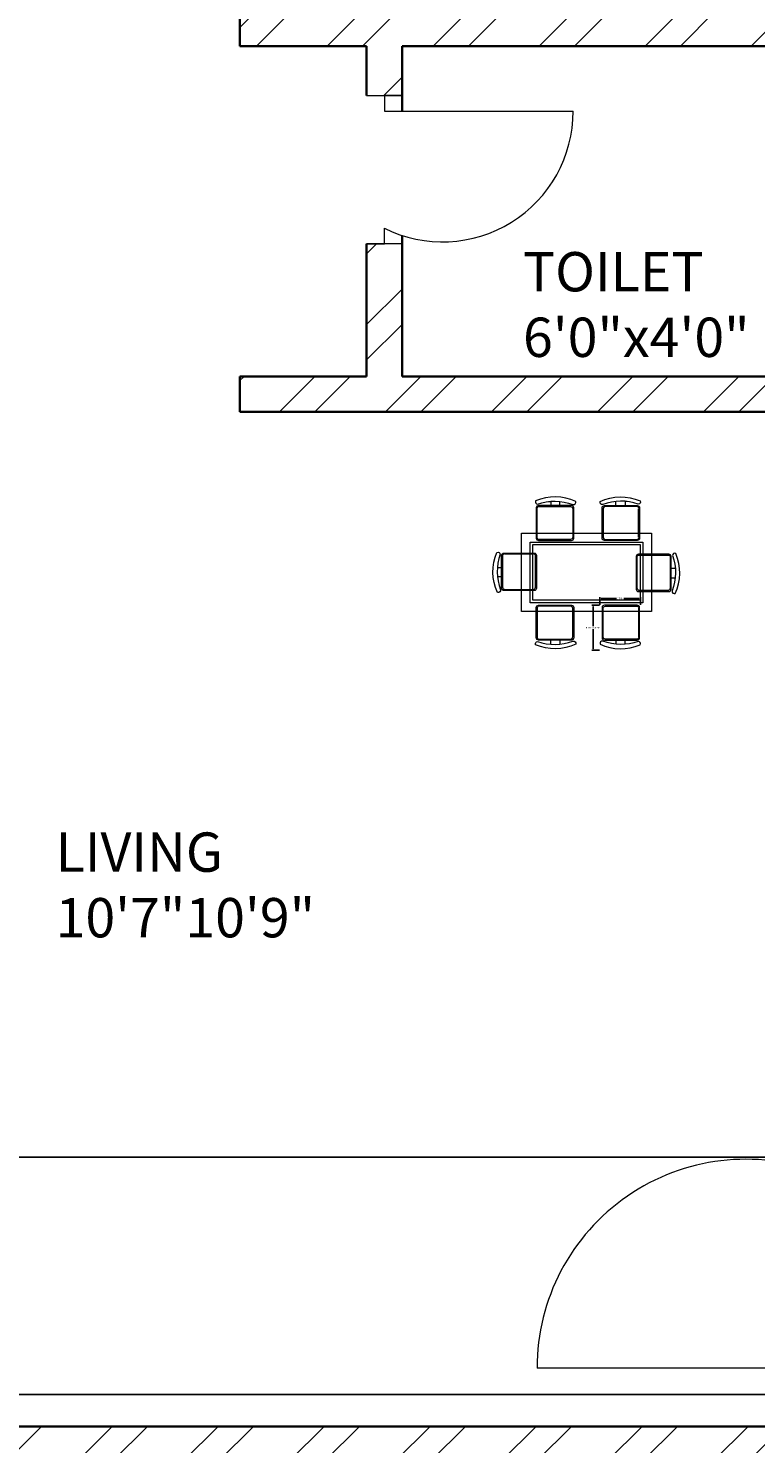
# Model space of a CAD drawing. Units: inches. Extents: x 1570 to 2186, y 1575 to 2421.
# Tile 7 of 10: x 1713 to 1806, y 2045 to 2225. Entities that reach past the tile are written whole.
import ezdxf

# ---------------------------------------------------------------- set-up
doc = ezdxf.new("R2010")
doc.units = ezdxf.units.IN
for name, color, linetype, lineweight in [('A-ANNO-DIMS', 2, 'Continuous', 18), ('A-AREA-IDEN', 7, 'Continuous', 18), ('A-DOOR', 201, 'Continuous', 18), ('A-FURN', 8, 'Continuous', 13), ('A-WALL', 7, 'Continuous', 35), ('A-WALL-PATT', 252, 'Continuous', 13)]:
    doc.layers.add(name, color=color, linetype=linetype, lineweight=lineweight)
doc.styles.get("Standard").update_dxf_attribs({"font": 'arial.ttf'})
doc.dimstyles.get("Standard").update_dxf_attribs({"dimtxt": 0.18, "dimasz": 0.18, "dimexe": 0.18, "dimexo": 0.0625, "dimgap": 0.09, "dimtad": 0, "dimtih": 1, "dimtoh": 1, "dimdec": 4, "dimzin": 0, "dimdsep": 46, "dimtxsty": 'Standard', "dimcen": 0.09, "dimadec": 0, "dimazin": 0, "dimtfac": 1, "dimtdec": 4, "dimtofl": 0, "dimtmove": 0, "dimatfit": 3, "dimfxl": 1, "dimtolj": 1, "dimtzin": 0, "dimarcsym": 0})

# ---------------------------------------------------------------- blocks, each defined once
blk = doc.blocks.new('TABLE-DINING')
for points in [[(0, 9.93), (16.54, 9.93), (16.54, 0), (0, 0)], [(0, 9.93), (16.54, 9.93), (16.54, 0), (0, 0)], [(1.1, 8.82), (15.44, 8.82), (15.44, 1.1), (1.1, 1.1)], [(1.1, 8.82), (15.44, 8.82), (15.44, 1.1), (1.1, 1.1)], [(1.43, 8.49), (15.11, 8.49), (15.11, 1.43), (1.43, 1.43)], [(1.43, 8.49), (15.11, 8.49), (15.11, 1.43), (1.43, 1.43)]]:
    blk.add_lwpolyline(points, close=True)
blk = doc.blocks.new('DINING-CHAIR-RH')
for points in [[(4.73, 1.1, 0.414214), (5.02, 1.39), (5.02, 5.24, 0.414214), (4.73, 5.53), (0.55, 5.53, 0.414214), (0.25, 5.24), (0.25, 1.39, 0.414214), (0.55, 1.1), (4.73, 1.1)], [(4.73, 1.1, 0.414214), (5.02, 1.39), (5.02, 5.24, 0.414214), (4.73, 5.53), (0.55, 5.53, 0.414214), (0.25, 5.24), (0.25, 1.39, 0.414214), (0.55, 1.1), (4.73, 1.1)], [(4.86, 0.92, -0.175809), (0.35, 0.96, 0.578392), (0.01, 0.58, 0.214524), (5.1, 0.51, 0.552014), (4.86, 0.92, -0.065079)], [(4.86, 0.92, -0.175809), (0.35, 0.96, 0.578392), (0.01, 0.58, 0.214524), (5.1, 0.51, 0.552014), (4.86, 0.92, -0.065079)], [(2.02, 1.1), (2.02, 0.57, -0.064759)], [(2.02, 1.1), (2.02, 0.57, -0.064759)]]:
    blk.add_lwpolyline(points, format="xyb")
blk.add_lwpolyline([(4.73, 1.23), (0.68, 1.23, -0.414214), (0.39, 1.53), (0.39, 5.11, -0.414214), (0.68, 5.4), (4.73, 5.4, -0.512069), (4.89, 5.11), (4.89, 1.53, -0.512069)], format="xyb", close=True)
blk.add_lwpolyline([(4.73, 1.23), (0.68, 1.23, -0.414214), (0.39, 1.53), (0.39, 5.11, -0.414214), (0.68, 5.4), (4.73, 5.4, -0.512069), (4.89, 5.11), (4.89, 1.53, -0.512069)], format="xyb", close=True)
blk.add_lwpolyline([(3.19, 0.56), (3.19, 1.1)])
blk.add_lwpolyline([(3.19, 0.56), (3.19, 1.1)])
blk = doc.blocks.new('*D20')
at = {"layer": 'A-ANNO-DIMS', "color": 0, "lineweight": -2, "transparency": 16777216}
for p, q in [((1785.77, 2151.55), (1784.79, 2151.55)), ((1784.97, 2151.37), (1784.97, 2148.87)), ((1784.97, 2146.01), (1784.97, 2148.51)), ((1785.77, 2145.83), (1784.79, 2145.83))]:
    blk.add_line(p, q, dxfattribs=at)
at = {"layer": 'A-ANNO-DIMS', "color": 0, "transparency": 16777216}
for points in [[(1784.94, 2151.37), (1785, 2151.37), (1784.97, 2151.55)], [(1784.94, 2146.01), (1785, 2146.01), (1784.97, 2145.83)]]:
    blk.add_solid(points, dxfattribs=at)
at = {"layer": 'Defpoints', "color": 0, "transparency": 16777216}
for p in [(1784.97, 2151.55), (1785.83, 2151.55), (1785.83, 2145.83)]:
    blk.add_point(p, dxfattribs=at)
at = {"layer": 'A-ANNO-DIMS', "color": 0, "transparency": 16777216, "insert": (1784.97, 2148.69), "char_height": 0.18, "attachment_point": 5}
blk.add_mtext('\\A1;RH CHAIR 6 TYP.', dxfattribs=at)
blk = doc.blocks.new('*D21')
at = {"layer": 'A-ANNO-DIMS', "color": 0, "lineweight": -2, "transparency": 16777216}
for p, q in [((1785.83, 2151.62), (1785.83, 2152.59)), ((1786.01, 2152.41), (1787.96, 2152.41)), ((1790.81, 2152.41), (1788.87, 2152.41)), ((1790.99, 2151.62), (1790.99, 2152.59))]:
    blk.add_line(p, q, dxfattribs=at)
at = {"layer": 'A-ANNO-DIMS', "color": 0, "transparency": 16777216}
for points in [[(1786.01, 2152.44), (1786.01, 2152.38), (1785.83, 2152.41)], [(1790.81, 2152.44), (1790.81, 2152.38), (1790.99, 2152.41)]]:
    blk.add_solid(points, dxfattribs=at)
at = {"layer": 'Defpoints', "color": 0, "transparency": 16777216}
for p in [(1790.99, 2152.41), (1785.83, 2151.55), (1790.99, 2151.55)]:
    blk.add_point(p, dxfattribs=at)
at = {"layer": 'A-ANNO-DIMS', "color": 0, "transparency": 16777216, "insert": (1788.41, 2152.41), "char_height": 0.18, "attachment_point": 5}
blk.add_mtext('\\A1;5 TYP.', dxfattribs=at)
blk = doc.blocks.new('*D42')
at = {"layer": 'A-ANNO-DIMS', "color": 0, "lineweight": -2, "transparency": 16777216}
for p, q in [((1913.53, 2081.37), (1603.11, 2081.37)), ((1603.29, 2081.19), (1603.29, 2066.47)), ((1603.29, 2051.39), (1603.29, 2066.11)), ((1913.53, 2051.21), (1603.11, 2051.21))]:
    blk.add_line(p, q, dxfattribs=at)
at = {"layer": 'A-ANNO-DIMS', "color": 0, "transparency": 16777216}
for points in [[(1603.26, 2081.19), (1603.32, 2081.19), (1603.29, 2081.37)], [(1603.26, 2051.39), (1603.32, 2051.39), (1603.29, 2051.21)]]:
    blk.add_solid(points, dxfattribs=at)
at = {"layer": 'Defpoints', "color": 0, "transparency": 16777216}
for p in [(1603.29, 2081.37), (1913.59, 2081.37), (1913.59, 2051.21)]:
    blk.add_point(p, dxfattribs=at)
at = {"layer": 'A-ANNO-DIMS', "color": 0, "transparency": 16777216, "insert": (1603.29, 2066.29), "char_height": 0.18, "attachment_point": 5}
blk.add_mtext('\\A1;30.165', dxfattribs=at)

msp = doc.modelspace()

# ---------------------------------------------------------------- hatches: boundary and pattern name
at = {"layer": 'A-WALL-PATT'}
h = msp.add_hatch(dxfattribs=at)
h.set_pattern_fill('ANSI32', color=256)
h.paths.add_polyline_path([(1762.0975, 2362.1492), (1757.5975, 2362.1492), (1757.5975, 2357.6492), (1709.1163, 2357.6492), (1709.1163, 2362.1492), (1704.6163, 2362.1492), (1704.6163, 2353.1492), (1740.0886, 2353.1492), (1740.0886, 2261.8115), (1744.5886, 2261.8115), (1744.5886, 2353.1492), (1762.0975, 2353.1492)])
h.paths.add_polyline_path([(1890.2592, 2362.1492), (1885.7592, 2362.1492), (1826.5975, 2362.1492), (1822.0975, 2362.1492), (1822.0975, 2353.1492), (1862.5886, 2353.1492), (1862.5886, 2227.1492), (1744.5886, 2227.1492), (1744.5886, 2229.5389), (1742.3386, 2229.5389), (1740.0886, 2229.5389), (1740.0886, 2222.6492), (1744.5886, 2222.6492), (1756.186, 2222.6492), (1756.186, 2216.3571), (1760.686, 2216.3571), (1760.686, 2222.6492), (1832.686, 2222.6492), (1832.686, 2212.5994), (1837.186, 2212.5994), (1837.186, 2222.6492), (1893.186, 2222.6492), (1893.186, 2212.5994), (1897.686, 2212.5994), (1897.686, 2222.6492), (1989.5886, 2222.6492), (1989.5886, 2227.1492), (1989.5886, 2232.6585), (1987.3386, 2232.6585), (1985.0886, 2232.6585), (1985.0886, 2227.1492), (1867.0886, 2227.1492), (1867.0886, 2353.1492), (1890.2592, 2353.1492)])
h.paths.add_polyline_path([(1644.0886, 2353.1492), (1668.6163, 2353.1492), (1668.6163, 2362.1492), (1664.1163, 2362.1492), (1664.1163, 2358.9932), (1664.1163, 2357.6492), (1639.5886, 2357.6492), (1639.5886, 2213.8746), (1644.0886, 2213.8746), (1644.0886, 2222.6492), (1692.0886, 2222.6492), (1692.0886, 2215.9343), (1696.5886, 2215.9343), (1696.5886, 2222.6492), (1696.5886, 2227.1492), (1644.0886, 2227.1492)])
h.paths.add_polyline_path([(2013.0435, 2362.1492), (2008.5435, 2362.1492), (2008.5435, 2357.6492), (1954.7592, 2357.6492), (1954.7592, 2362.1492), (1950.2592, 2362.1492), (1950.2592, 2353.1492), (1985.0886, 2353.1492), (1985.0886, 2260.8534), (1989.5886, 2260.8534), (1989.5886, 2353.1492), (2013.0435, 2353.1492)])
h.paths.add_polyline_path([(2090.0886, 2357.6492), (2053.5435, 2357.6492), (2053.5435, 2362.1492), (2049.0435, 2362.1492), (2049.0435, 2353.1492), (2085.5886, 2353.1492), (2085.5886, 2227.1492), (2033.0886, 2227.1492), (2033.0886, 2222.6492), (2033.0886, 2214.4464), (2037.5886, 2214.4464), (2037.5886, 2222.6492), (2085.5886, 2222.6492), (2085.5886, 2212.4409), (2090.0886, 2212.4409)])
h.paths.add_polyline_path([(2090.0886, 2188.4409), (2087.8386, 2188.4409), (2085.5886, 2188.4409), (2085.5886, 2180.6492), (2037.5886, 2180.6492), (2037.5886, 2196.7956), (2033.0886, 2196.7956), (2033.0886, 2176.1492), (2037.5886, 2176.1492), (2045.0886, 2176.1492), (2045.0886, 2169.8988), (2049.5886, 2169.8988), (2049.5886, 2176.1492), (2085.5886, 2176.1492), (2085.5886, 2167.785), (2090.0886, 2167.785)])
h.paths.add_polyline_path([(2049.5886, 2147.4502), (2047.3386, 2147.4502), (2045.0886, 2147.4502), (2045.0886, 2124.4703), (2049.5886, 2124.4703)])
h.paths.add_polyline_path([(2090.0886, 2047.1492), (2049.5886, 2047.1492), (2049.5886, 2064.4703), (2045.0886, 2064.4703), (2045.0886, 2047.1492), (1918.0886, 2047.1492), (1918.0886, 2051.2061), (1913.5886, 2051.2061), (1913.5886, 2047.1492), (1913.5886, 2036.6872), (1918.0886, 2036.6872), (1918.0886, 2042.7492), (2045.0886, 2042.7492), (2045.0886, 2027.0686), (2049.5886, 2027.0686), (2049.5886, 2042.7492), (2090.0886, 2042.7492)])
h.paths.add_polyline_path([(1918.0886, 2005.9338), (1915.8386, 2005.9338), (1913.5886, 2005.9338), (1913.5886, 1913.7492), (1918.0886, 1913.7492)])
h.paths.add_polyline_path([(2090.0886, 1913.7492), (2049.5886, 1913.7492), (2045.0886, 1913.7492), (2033.0886, 1913.7492), (2033.0886, 1909.2492), (2033.0886, 1900.9803), (2037.5886, 1900.9803), (2037.5886, 1909.2492), (2085.5886, 1909.2492), (2085.5886, 1861.2492), (2037.5886, 1861.2492), (2037.5886, 1880.0859), (2033.0886, 1880.0859), (2033.0886, 1856.7492), (2085.5886, 1856.7492), (2085.5886, 1730.7492), (2054.2483, 1730.7492), (2054.2483, 1721.7492), (2058.7483, 1721.7492), (2058.7483, 1726.2492), (2090.0886, 1726.2492)])
h.paths.add_polyline_path([(2049.5886, 1967.0686), (2045.0886, 1967.0686), (2045.0886, 1913.7492), (2049.5886, 1913.7492)])
h.paths.add_polyline_path([(1989.5886, 1824.1695), (1987.3386, 1824.1695), (1985.0886, 1824.1695), (1985.0886, 1730.7492), (1989.5886, 1730.7492)])
h.paths.add_polyline_path([(1989.5886, 1861.2492), (1974.9963, 1861.2492), (1974.9963, 1865.9306), (1972.7463, 1865.9306), (1970.4963, 1865.9306), (1970.4963, 1861.2492), (1898.4963, 1861.2492), (1898.4963, 1874.2999), (1893.9963, 1874.2999), (1893.9963, 1861.2492), (1890.5886, 1861.2492), (1837.9963, 1861.2492), (1837.9963, 1874.3159), (1833.4963, 1874.3159), (1833.4963, 1861.2492), (1761.4963, 1861.2492), (1761.4963, 1865.0209), (1759.2463, 1865.0209), (1756.9963, 1865.0209), (1756.9963, 1861.2492), (1740.0886, 1861.2492), (1740.0886, 1856.7492), (1740.0886, 1850.7206), (1744.5886, 1850.7206), (1744.5886, 1856.7492), (1985.0886, 1856.7492), (1985.0886, 1851.0804), (1989.5886, 1851.0804), (1989.5886, 1856.7492)])
h.paths.add_polyline_path([(1989.5886, 1913.7492), (1740.0886, 1913.7492), (1740.0886, 1909.2492), (1756.9963, 1909.2492), (1756.9963, 1890.279), (1761.4963, 1890.279), (1761.4963, 1909.2492), (1833.4963, 1909.2492), (1833.4963, 1898.3159), (1837.9963, 1898.3159), (1837.9963, 1909.2492), (1890.5886, 1909.2492), (1893.9963, 1909.2492), (1893.9963, 1898.2999), (1898.4963, 1898.2999), (1898.4963, 1909.2492), (1970.4963, 1909.2492), (1970.4963, 1886.9887), (1974.9963, 1886.9887), (1974.9963, 1909.2492), (1989.5886, 1909.2492)])
h.paths.add_polyline_path([(1893.7344, 1730.7492), (1867.0886, 1730.7492), (1867.0886, 1856.7492), (1862.5886, 1856.7492), (1862.5886, 1730.7492), (1824.0492, 1730.7492), (1824.0492, 1721.7492), (1893.7344, 1721.7492)])
h.paths.add_polyline_path([(2018.2483, 1730.7492), (1953.7344, 1730.7492), (1953.7344, 1721.7492), (1958.2344, 1721.7492), (1958.2344, 1726.2492), (2013.7483, 1726.2492), (2013.7483, 1721.7492), (2018.2483, 1721.7492)])
h.paths.add_polyline_path([(1768.5492, 1730.7492), (1764.0492, 1730.7492), (1744.5886, 1730.7492), (1744.5886, 1819.4364), (1742.3386, 1819.4364), (1740.0886, 1819.4364), (1740.0886, 1730.7492), (1697.3801, 1730.7492), (1697.3801, 1721.7492), (1701.8801, 1721.7492), (1701.8801, 1726.2492), (1764.0492, 1726.2492), (1764.0492, 1721.7492), (1768.5492, 1721.7492)])
h.paths.add_polyline_path([(1644.0886, 1856.7492), (1639.5886, 1856.7492), (1639.5886, 1726.2492), (1657.0315, 1726.2492), (1657.0315, 1721.7492), (1661.3801, 1721.7492), (1661.3801, 1730.7492), (1644.0886, 1730.7492)])
h.paths.add_polyline_path([(1696.5886, 1876.1809), (1692.0886, 1876.1809), (1692.0886, 1861.2492), (1684.5886, 1861.2492), (1644.0886, 1861.2492), (1644.0886, 1909.2492), (1692.0886, 1909.2492), (1692.0886, 1900.3394), (1696.5886, 1900.3394), (1696.5886, 1913.7492), (1684.5886, 1913.7492), (1684.5886, 1920.2115), (1682.3386, 1920.2115), (1680.0886, 1920.2115), (1680.0886, 1913.7492), (1639.5886, 1913.7492), (1639.5886, 1856.7492), (1684.5886, 1856.7492), (1692.0886, 1856.7492), (1696.5886, 1856.7492)])
h.paths.add_polyline_path([(1684.5886, 2042.7492), (1811.5886, 2042.7492), (1811.5886, 2038.2991), (1816.0886, 2038.2991), (1816.0886, 2042.7492), (1816.0886, 2052.5708), (1813.8386, 2052.5708), (1811.5886, 2052.5708), (1811.5886, 2047.1492), (1684.5886, 2047.1492), (1684.5886, 2064.4703), (1680.0886, 2064.4703), (1680.0886, 2047.1492), (1639.5886, 2047.1492), (1639.5886, 2042.7492), (1680.0886, 2042.7492), (1680.0886, 2024.0762), (1684.5886, 2024.0762)])
h.paths.add_polyline_path([(1684.5886, 1964.0762), (1680.0886, 1964.0762), (1680.0886, 1944.6145), (1684.5886, 1944.6145)])
h.paths.add_polyline_path([(1816.0886, 1973.7492), (1876.0886, 1973.7492), (1876.0886, 1959.17), (1880.5886, 1959.17), (1880.5886, 1973.7492), (1880.5886, 1978.2492), (1816.0886, 1978.2492), (1816.0886, 2005.9338), (1813.8386, 2005.9338), (1811.5886, 2005.9338), (1811.5886, 1913.7492), (1816.0886, 1913.7492)])
h.paths.add_polyline_path([(1837.186, 2180.6492), (1837.186, 2188.5994), (1834.936, 2188.5994), (1832.686, 2188.5994), (1832.686, 2180.6492), (1760.686, 2180.6492), (1760.686, 2197.4807), (1756.186, 2197.4807), (1756.186, 2180.6492), (1744.5886, 2180.6492), (1740.0886, 2180.6492), (1740.0886, 2176.1492), (1837.186, 2176.1492)])
h.paths.add_polyline_path([(1974.186, 2196.8744), (1971.936, 2196.8744), (1969.686, 2196.8744), (1969.686, 2180.6492), (1897.686, 2180.6492), (1897.686, 2188.5994), (1895.436, 2188.5994), (1893.186, 2188.5994), (1893.186, 2180.6492), (1893.186, 2176.1492), (1974.186, 2176.1492)])
h.paths.add_polyline_path([(1918.0886, 2176.1492), (1913.5886, 2176.1492), (1913.5886, 2081.3709), (1918.0886, 2081.3709)])
h.paths.add_polyline_path([(1816.0886, 2176.1492), (1811.5886, 2176.1492), (1811.5886, 2081.3709), (1816.0886, 2081.3709)])
h.paths.add_polyline_path([(1684.5886, 2150.4939), (1682.3386, 2150.4939), (1680.0886, 2150.4939), (1680.0886, 2124.4703), (1684.5886, 2124.4703)])
h.paths.add_polyline_path([(1696.5886, 2180.6492), (1696.5886, 2197.4701), (1692.0886, 2197.4701), (1692.0886, 2180.6492), (1644.0886, 2180.6492), (1644.0886, 2189.8746), (1641.8386, 2189.8746), (1639.5886, 2189.8746), (1639.5886, 2169.814), (1644.0886, 2169.814), (1644.0886, 2176.1492), (1680.0886, 2176.1492), (1680.0886, 2171.7002), (1684.5886, 2171.7002), (1684.5886, 2176.1492), (1696.5886, 2176.1492)])

# ---------------------------------------------------------------- linework, layer by layer
at = {"layer": 'A-DOOR'}
for p, q in [((1756.186, 2216.3571), (1760.686, 2216.3571)), ((1760.686, 2216.3571), (1758.436, 2216.3571)), ((1758.436, 2216.3571), (1758.436, 2214.3571)), ((1758.436, 2214.3571), (1782.436, 2214.3571)), ((1758.436, 2197.4807), (1758.436, 2199.4807)), ((1760.686, 2197.4807), (1756.186, 2197.4807)), ((1756.186, 2197.4807), (1758.436, 2197.4807)), ((1813.8386, 2054.5708), (1777.8386, 2054.5708))]:
    msp.add_line(p, q, dxfattribs=at)
for centre, radius, start, end in [((1765.8254, 2214.3571), 16.6106, 243.585434, 0), ((1804.381, 2054.5708), 26.5423, 69.125341, 180)]:
    msp.add_arc(centre, radius, start, end, dxfattribs=at)
at = {"layer": 'A-FURN'}
for points in [[(1777.9063, 2164.4009, -0.17580919), (1782.4121, 2164.3668, 0.57839206), (1782.7535, 2164.7421, 0.21452438), (1777.6673, 2164.8103, 0.55201397), (1777.9063, 2164.4009, -0.06507904)], [(1777.9063, 2164.4007, -0.17580919), (1782.4121, 2164.3666, 0.57839206), (1782.7535, 2164.7419, 0.21452438), (1777.6673, 2164.8102, 0.55201397), (1777.9063, 2164.4007, -0.06507904)], [(1786.2054, 2164.3668, -0.57839206), (1785.8641, 2164.7421, -0.21452438), (1790.9502, 2164.8103, -0.55201397), (1790.7113, 2164.4009, 0.1758092), (1786.2054, 2164.3668)], [(1786.2054, 2164.3666, -0.57839206), (1785.8641, 2164.7419, -0.21452438), (1790.9502, 2164.8102, -0.55201397), (1790.7113, 2164.4007, 0.1758092), (1786.2054, 2164.3666)], [(1782.2209, 2164.22), (1778.0379, 2164.22, 0.41421356), (1777.7452, 2163.9274), (1777.7452, 2160.0811, 0.41421356), (1778.0379, 2159.7885), (1782.2209, 2159.7885, 0.41421356), (1782.5136, 2160.0811), (1782.5136, 2163.9274, 0.41421356), (1782.2209, 2164.22)], [(1782.221, 2164.2199), (1778.0379, 2164.2199, 0.41421356), (1777.7452, 2163.9272), (1777.7452, 2160.081, 0.41421356), (1778.0379, 2159.7883), (1782.221, 2159.7883, 0.41421356), (1782.5136, 2160.081), (1782.5136, 2163.9272, 0.41421356), (1782.221, 2164.2199)], [(1780.7516, 2164.22), (1780.7516, 2164.7491, -0.06475861)], [(1780.7517, 2164.2199), (1780.7517, 2164.7489, -0.06475861)], [(1790.5796, 2164.22, -0.41421356), (1790.8723, 2163.9274), (1790.8723, 2160.0811, -0.41421356), (1790.5796, 2159.7885), (1786.3966, 2159.7885, -0.41421356), (1786.1039, 2160.0811), (1786.1039, 2163.9274, -0.41421356), (1786.3966, 2164.22), (1790.5796, 2164.22)], [(1790.5797, 2164.2199, -0.41421356), (1790.8723, 2163.9272), (1790.8723, 2160.081, -0.41421356), (1790.5797, 2159.7883), (1786.3966, 2159.7883, -0.41421356), (1786.104, 2160.081), (1786.104, 2163.9272, -0.41421356), (1786.3966, 2164.2199), (1790.5797, 2164.2199)], [(1787.8659, 2164.22), (1787.8659, 2164.7491, 0.06475861)], [(1787.8659, 2164.2199), (1787.8659, 2164.7489, 0.06475861)], [(1773.1923, 2153.52, -0.57839206), (1772.817, 2153.1786, -0.21452438), (1772.7487, 2158.2648, -0.55201397), (1773.1582, 2158.0258, 0.17580937), (1773.1923, 2153.52)], [(1773.1923, 2153.5198, -0.57839206), (1772.817, 2153.1785, -0.21452438), (1772.7487, 2158.2646, -0.55201397), (1773.1582, 2158.0256, 0.17580937), (1773.1923, 2153.5198)], [(1773.339, 2157.8942, -0.41421356), (1773.6317, 2158.1869), (1777.4779, 2158.1869, -0.41421356), (1777.7706, 2157.8942), (1777.7706, 2153.7112, -0.41421356), (1777.4779, 2153.4185), (1773.6317, 2153.4185, -0.41421356), (1773.339, 2153.7112), (1773.339, 2157.8942)], [(1773.3391, 2157.894, -0.41421356), (1773.6317, 2158.1867), (1777.4779, 2158.1867, -0.41421356), (1777.7706, 2157.894), (1777.7706, 2153.711, -0.41421356), (1777.4779, 2153.4183), (1773.6317, 2153.4183, -0.41421356), (1773.3391, 2153.711), (1773.3391, 2157.894)], [(1794.8798, 2157.7509, 0.41421356), (1794.5872, 2158.0436), (1790.7409, 2158.0436, 0.41421356), (1790.4483, 2157.7509), (1790.4483, 2153.5679, 0.41421356), (1790.7409, 2153.2752), (1794.5872, 2153.2752, 0.41421356), (1794.8798, 2153.5679), (1794.8798, 2157.7509)], [(1794.8798, 2157.7508, 0.41421356), (1794.5872, 2158.0434), (1790.7409, 2158.0434, 0.41421356), (1790.4483, 2157.7508), (1790.4483, 2153.5677, 0.41421356), (1790.7409, 2153.2751), (1794.5872, 2153.2751, 0.41421356), (1794.8798, 2153.5677), (1794.8798, 2157.7508)], [(1795.0607, 2157.8826, -0.17580919), (1795.0265, 2153.3767, 0.57839206), (1795.4019, 2153.0354, 0.21452438), (1795.4701, 2158.1215, 0.55201397), (1795.0607, 2157.8826, -0.06507904)], [(1795.0607, 2157.8824, -0.17580919), (1795.0266, 2153.3766, 0.57839206), (1795.4019, 2153.0352, 0.21452438), (1795.4701, 2158.1213, 0.55201397), (1795.0607, 2157.8824, -0.06507904)], [(1773.339, 2155.1805), (1772.81, 2155.1805, 0.06475861)], [(1773.3391, 2155.1803), (1772.81, 2155.1803, 0.06475861)], [(1794.8798, 2155.0372), (1795.4089, 2155.0372, -0.06475861)], [(1794.8798, 2155.037), (1795.4089, 2155.037, -0.06475861)], [(1782.2209, 2147.1226), (1778.0379, 2147.1226, -0.41421356), (1777.7452, 2147.4152), (1777.7452, 2151.2614, -0.41421356), (1778.0379, 2151.5541), (1782.2209, 2151.5541, -0.41421356), (1782.5136, 2151.2614), (1782.5136, 2147.4152, -0.41421356), (1782.2209, 2147.1226)], [(1782.221, 2147.1224), (1778.0379, 2147.1224, -0.41421356), (1777.7452, 2147.415), (1777.7452, 2151.2613, -0.41421356), (1778.0379, 2151.5539), (1782.221, 2151.5539, -0.41421356), (1782.5136, 2151.2613), (1782.5136, 2147.415, -0.41421356), (1782.221, 2147.1224)], [(1782.4121, 2146.9758, -0.57839206), (1782.7535, 2146.6005, -0.21452438), (1777.6673, 2146.5322, -0.55201397), (1777.9063, 2146.9417, 0.17580929), (1782.4121, 2146.9758)], [(1782.4121, 2146.9757, -0.57839206), (1782.7535, 2146.6003, -0.21452438), (1777.6673, 2146.5321, -0.55201397), (1777.9063, 2146.9415, 0.17580929), (1782.4121, 2146.9757)], [(1780.7516, 2147.1226), (1780.7516, 2146.5935, 0.06475861)], [(1780.7517, 2147.1224), (1780.7517, 2146.5934, 0.06475861)]]:
    msp.add_lwpolyline(points, format="xyb", dxfattribs=at)
for points in [[(1778.0397, 2164.0882), (1782.0891, 2164.0882, -0.41421356), (1782.3818, 2163.7955), (1782.3818, 2160.213, -0.41421356), (1782.0891, 2159.9203), (1778.0397, 2159.9203, -0.51206948), (1777.8771, 2160.213), (1777.8771, 2163.7955, -0.51206948)], [(1778.0397, 2164.088), (1782.0891, 2164.088, -0.41421356), (1782.3818, 2163.7954), (1782.3818, 2160.2128, -0.41421356), (1782.0891, 2159.9202), (1778.0397, 2159.9202, -0.51206948), (1777.8771, 2160.2128), (1777.8771, 2163.7954, -0.51206948)], [(1790.5779, 2164.0882), (1786.5284, 2164.0882, 0.41421356), (1786.2358, 2163.7955), (1786.2358, 2160.213, 0.41421356), (1786.5284, 2159.9203), (1790.5779, 2159.9203, 0.51206948), (1790.7405, 2160.213), (1790.7405, 2163.7955, 0.51206948)], [(1790.5779, 2164.088), (1786.5284, 2164.088, 0.41421356), (1786.2358, 2163.7954), (1786.2358, 2160.2128, 0.41421356), (1786.5284, 2159.9202), (1790.5779, 2159.9202, 0.51206948), (1790.7405, 2160.2128), (1790.7405, 2163.7954, 0.51206948)], [(1773.4709, 2157.8924), (1773.4709, 2153.843, 0.41421356), (1773.7635, 2153.5503), (1777.3461, 2153.5503, 0.41421356), (1777.6387, 2153.843), (1777.6387, 2157.8924, 0.51206948), (1777.3461, 2158.055), (1773.7635, 2158.055, 0.51206948)], [(1773.4709, 2157.8923), (1773.4709, 2153.8428, 0.41421356), (1773.7635, 2153.5502), (1777.3461, 2153.5502, 0.41421356), (1777.6388, 2153.8428), (1777.6388, 2157.8923, 0.51206948), (1777.3461, 2158.0548), (1773.7635, 2158.0548, 0.51206948)], [(1794.748, 2157.7492), (1794.748, 2153.6997, -0.41421356), (1794.4553, 2153.4071), (1790.8728, 2153.4071, -0.41421356), (1790.5801, 2153.6997), (1790.5801, 2157.7492, -0.51206948), (1790.8728, 2157.9118), (1794.4553, 2157.9118, -0.51206948)], [(1794.748, 2157.749), (1794.748, 2153.6996, -0.41421356), (1794.4553, 2153.4069), (1790.8728, 2153.4069, -0.41421356), (1790.5801, 2153.6996), (1790.5801, 2157.749, -0.51206948), (1790.8728, 2157.9116), (1794.4553, 2157.9116, -0.51206948)], [(1778.0397, 2147.2544), (1782.0891, 2147.2544, 0.41421356), (1782.3818, 2147.547), (1782.3818, 2151.1296, 0.41421356), (1782.0891, 2151.4223), (1778.0397, 2151.4223, 0.51206948), (1777.8771, 2151.1296), (1777.8771, 2147.547, 0.51206948)], [(1778.0397, 2147.2542), (1782.0891, 2147.2542, 0.41421356), (1782.3818, 2147.5469), (1782.3818, 2151.1294, 0.41421356), (1782.0891, 2151.4221), (1778.0397, 2151.4221, 0.51206948), (1777.8771, 2151.1294), (1777.8771, 2147.5469, 0.51206948)]]:
    msp.add_lwpolyline(points, format="xyb", close=True, dxfattribs=at)
for points in [[(1779.5807, 2164.7587), (1779.5807, 2164.22)], [(1779.5808, 2164.7585), (1779.5808, 2164.2199)], [(1789.0368, 2164.7587), (1789.0368, 2164.22)], [(1789.0368, 2164.7585), (1789.0368, 2164.2199)], [(1772.8004, 2156.3514), (1773.339, 2156.3514)], [(1772.8004, 2156.3512), (1773.3391, 2156.3512)], [(1795.4185, 2156.2081), (1794.8798, 2156.2081)], [(1795.4185, 2156.2079), (1794.8798, 2156.2079)], [(1779.5807, 2146.5839), (1779.5807, 2147.1226)], [(1779.5808, 2146.5837), (1779.5808, 2147.1224)]]:
    msp.add_lwpolyline(points, dxfattribs=at)
at = {"layer": 'A-WALL'}
for p, q in [((1740.0886, 2229.5389), (1740.0886, 2222.6492)), ((1744.5886, 2222.6492), (1740.0886, 2222.6492)), ((1744.5886, 2222.6492), (1756.186, 2222.6492)), ((1756.186, 2222.6492), (1756.186, 2216.3571)), ((1760.686, 2214.3571), (1760.686, 2222.6492)), ((1760.686, 2222.6492), (1832.686, 2222.6492)), ((1756.186, 2197.4807), (1756.186, 2180.6492)), ((1760.686, 2180.6492), (1760.686, 2198.5617)), ((1740.0886, 2180.6492), (1740.0886, 2176.1492)), ((1744.5886, 2180.6492), (1740.0886, 2180.6492)), ((1744.5886, 2180.6492), (1756.186, 2180.6492)), ((1760.686, 2180.6492), (1832.686, 2180.6492)), ((1740.0886, 2176.1492), (1837.186, 2176.1492)), ((1684.5886, 2047.1492), (1811.5886, 2047.1492)), ((1811.5886, 2047.1492), (1684.5886, 2047.1492))]:
    msp.add_line(p, q, dxfattribs=at)

# ---------------------------------------------------------------- block references
at = {"layer": 'A-FURN'}
for name, p in [('TABLE-DINING', (1775.8597, 2150.7614)), ('DINING-CHAIR-RH', (1785.8507, 2146.0204))]:
    msp.add_blockref(name, p, dxfattribs=at)

# ---------------------------------------------------------------- texts
at = {"layer": 'A-AREA-IDEN', "char_height": 5, "attachment_point": 1}
for s, width, insert in [('TOILET\\P6\'0"x4\'0"', 64.70649, (1776.0579, 2196.4511)), ('LIVING\\P10\'7"10\'9"', 223.088706, (1716.6592, 2122.6589))]:
    msp.add_mtext_dynamic_manual_height_columns(s, width=width, gutter_width=12.5, heights=[0], dxfattribs=dict(at, insert=insert))

# ---------------------------------------------------------------- dimensions: what is measured, and where the dimension line sits
at = {"layer": 'A-ANNO-DIMS'}
dim = msp.add_linear_dim(base=(1790.9947, 2152.4133), p1=(1785.8321, 2151.5541), p2=(1790.9947, 2151.5541), text='<> TYP.', dimstyle='Standard', override={"dimdec": 0, "dimlfac": 1, "dimrnd": 0, "dimzin": 0, "dimdsep": 46, "dimlunit": 2}, dxfattribs=at)
dim.commit()
dim.dimension.update_dxf_attribs({"geometry": '*D21', "text_midpoint": (1788.4134, 2152.4133)})
dim = msp.add_linear_dim(base=(1784.9729, 2151.5541), p1=(1785.8321, 2145.8264), p2=(1785.8321, 2151.5541), angle=90, text='RH CHAIR <> TYP.', dimstyle='Standard', override={"dimdec": 0, "dimlfac": 1, "dimrnd": 0, "dimzin": 0, "dimdsep": 46, "dimlunit": 2}, dxfattribs=at)
dim.commit()
dim.dimension.update_dxf_attribs({"geometry": '*D20', "text_midpoint": (1784.9729, 2148.6902)})
dim = msp.add_linear_dim(base=(1603.2886, 2081.3709), p1=(1913.5886, 2051.2061), p2=(1913.5886, 2081.3709), angle=90, dimstyle='Standard', override={"dimdec": 3, "dimlfac": 1, "dimrnd": 0, "dimzin": 0, "dimdsep": 46, "dimlunit": 2}, dxfattribs=at)
dim.commit()
dim.dimension.update_dxf_attribs({"geometry": '*D42', "text_midpoint": (1603.2886, 2066.2885)})

doc.saveas('drawing.dxf')
